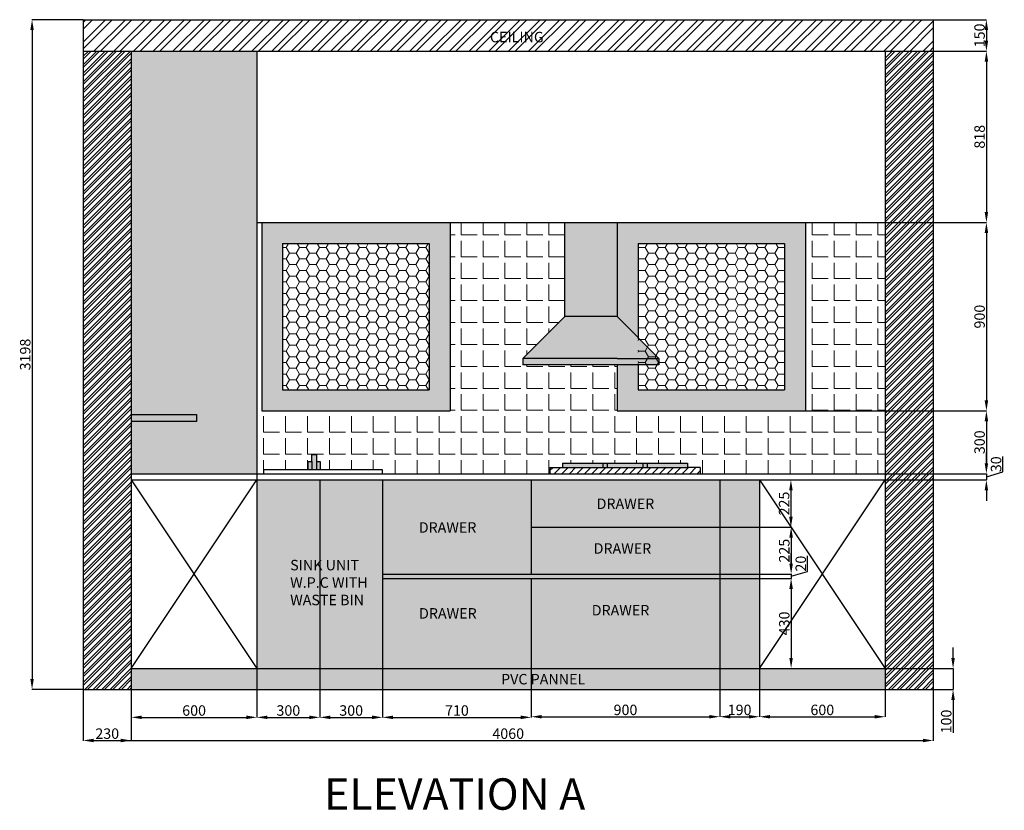
# Model space of a CAD drawing. Units: millimetres. Extents: x 4283 to 9420, y -2853 to 5191.
# Tile 1 of 2: x 4283 to 8985, y -2853 to 922. Entities that reach past the tile are written whole.
import ezdxf

# ---------------------------------------------------------------- set-up
doc = ezdxf.new("R2010")
doc.units = ezdxf.units.MM
for name, color, linetype, lineweight in [('A-ANNO-DIMS', 2, 'Continuous', 18), ('A-ANNO-TEXT', 7, 'Continuous', 18), ('A-ELEV', 7, 'Continuous', 25), ('A-ELEV-PATT', 252, 'Continuous', 13)]:
    doc.layers.add(name, color=color, linetype=linetype, lineweight=lineweight)
doc.styles.get("Standard").update_dxf_attribs({"font": 'arial.ttf'})
doc.dimstyles.new('ISO-25', dxfattribs={"dimtxt": 50, "dimasz": 50, "dimexe": 1.25, "dimexo": 0.625, "dimtad": 1, "dimdec": 0, "dimtxsty": 'Standard', "dimcen": 2.5, "dimclrd": 4, "dimclre": 4, "dimclrt": 4, "dimadec": 0, "dimazin": 0, "dimtfac": 1, "dimtdec": 0, "dimtmove": 0, "dimatfit": 3, "dimfxl": 1, "dimarcsym": 0})

# ---------------------------------------------------------------- blocks, each defined once
blk = doc.blocks.new('*D20')
at = {"layer": 'A-ANNO-DIMS', "color": 0, "lineweight": -2, "transparency": 16777216}
for p, q in [((8647.1, 922.3), (8901.2, 922.3)), ((8900, 872.3), (8900, 822.3)), ((8647.1, 772.3), (8901.2, 772.3))]:
    blk.add_line(p, q, dxfattribs=at)
at = {"layer": 'A-ANNO-DIMS', "color": 0, "transparency": 16777216}
for points in [[(8891.7, 872.3), (8908.3, 872.3), (8900, 922.3)], [(8891.7, 822.3), (8908.3, 822.3), (8900, 772.3)]]:
    blk.add_solid(points, dxfattribs=at)
at = {"layer": 'Defpoints', "color": 0, "transparency": 16777216}
for p in [(8646.4, 922.3), (8646.4, 772.3), (8900, 772.3)]:
    blk.add_point(p, dxfattribs=at)
at = {"layer": 'A-ANNO-DIMS', "color": 0, "transparency": 16777216, "insert": (8873.8, 847.3), "char_height": 50, "attachment_point": 5, "rotation": 90}
blk.add_mtext('150', dxfattribs=at)
blk = doc.blocks.new('*D21')
at = {"layer": 'A-ANNO-DIMS', "color": 0, "lineweight": -2, "transparency": 16777216}
for p, q in [((8647.1, 772.3), (8901.2, 772.3)), ((8900, 722.3), (8900, 4.3)), ((8417.1, -45.7), (8901.2, -45.7))]:
    blk.add_line(p, q, dxfattribs=at)
at = {"layer": 'A-ANNO-DIMS', "color": 0, "transparency": 16777216}
for points in [[(8891.7, 722.3), (8908.3, 722.3), (8900, 772.3)], [(8891.7, 4.3), (8908.3, 4.3), (8900, -45.7)]]:
    blk.add_solid(points, dxfattribs=at)
at = {"layer": 'Defpoints', "color": 0, "transparency": 16777216}
for p in [(8646.4, 772.3), (8416.4, -45.7), (8900, -45.7)]:
    blk.add_point(p, dxfattribs=at)
at = {"layer": 'A-ANNO-DIMS', "color": 0, "transparency": 16777216, "insert": (8873.8, 363.3), "char_height": 50, "attachment_point": 5, "rotation": 90}
blk.add_mtext('818', dxfattribs=at)
blk = doc.blocks.new('*D22')
at = {"layer": 'A-ANNO-DIMS', "color": 0, "lineweight": -2, "transparency": 16777216}
for p, q in [((8417.1, -45.7), (8901.2, -45.7)), ((8900, -95.7), (8900, -895.7)), ((8036.9, -945.7), (8901.2, -945.7))]:
    blk.add_line(p, q, dxfattribs=at)
at = {"layer": 'A-ANNO-DIMS', "color": 0, "transparency": 16777216}
for points in [[(8891.7, -95.7), (8908.3, -95.7), (8900, -45.7)], [(8891.7, -895.7), (8908.3, -895.7), (8900, -945.7)]]:
    blk.add_solid(points, dxfattribs=at)
at = {"layer": 'Defpoints', "color": 0, "transparency": 16777216}
for p in [(8416.4, -45.7), (8036.3, -945.7), (8900, -945.7)]:
    blk.add_point(p, dxfattribs=at)
at = {"layer": 'A-ANNO-DIMS', "color": 0, "transparency": 16777216, "insert": (8873.8, -495.7), "char_height": 50, "attachment_point": 5, "rotation": 90}
blk.add_mtext('900', dxfattribs=at)
blk = doc.blocks.new('*D23')
at = {"layer": 'A-ANNO-DIMS', "color": 0, "lineweight": -2, "transparency": 16777216}
for p, q in [((8036.9, -945.7), (8901.2, -945.7)), ((8900, -995.7), (8900, -1195.7)), ((8417.1, -1245.7), (8901.2, -1245.7))]:
    blk.add_line(p, q, dxfattribs=at)
at = {"layer": 'A-ANNO-DIMS', "color": 0, "transparency": 16777216}
for points in [[(8891.7, -995.7), (8908.3, -995.7), (8900, -945.7)], [(8891.7, -1195.7), (8908.3, -1195.7), (8900, -1245.7)]]:
    blk.add_solid(points, dxfattribs=at)
at = {"layer": 'Defpoints', "color": 0, "transparency": 16777216}
for p in [(8036.3, -945.7), (8416.4, -1245.7), (8900, -1245.7)]:
    blk.add_point(p, dxfattribs=at)
at = {"layer": 'A-ANNO-DIMS', "color": 0, "transparency": 16777216, "insert": (8873.8, -1095.7), "char_height": 50, "attachment_point": 5, "rotation": 90}
blk.add_mtext('300', dxfattribs=at)
blk = doc.blocks.new('*D24')
at = {"layer": 'A-ANNO-DIMS', "color": 0, "lineweight": -2, "transparency": 16777216}
for p, q in [((8900, -1195.7), (8900, -1145.7)), ((8978.8, -1237.1), (8978.8, -1164.4)), ((8417.1, -1245.7), (8901.2, -1245.7)), ((8900, -1260.7), (8978.8, -1237.1)), ((8900, -1245.7), (8900, -1275.7)), ((8900, -1245.7), (8900, -1275.7)), ((8417.1, -1275.7), (8901.2, -1275.7)), ((8900, -1325.7), (8900, -1375.7))]:
    blk.add_line(p, q, dxfattribs=at)
at = {"layer": 'A-ANNO-DIMS', "color": 0, "transparency": 16777216}
for points in [[(8891.7, -1195.7), (8908.3, -1195.7), (8900, -1245.7)], [(8891.7, -1325.7), (8908.3, -1325.7), (8900, -1275.7)]]:
    blk.add_solid(points, dxfattribs=at)
at = {"layer": 'Defpoints', "color": 0, "transparency": 16777216}
for p in [(8416.4, -1245.7), (8416.4, -1275.7), (8900, -1275.7)]:
    blk.add_point(p, dxfattribs=at)
at = {"layer": 'A-ANNO-DIMS', "color": 0, "transparency": 16777216, "insert": (8952.7, -1200.8), "char_height": 50, "attachment_point": 5, "rotation": 90}
blk.add_mtext('30', dxfattribs=at)
blk = doc.blocks.new('*D25')
at = {"layer": 'A-ANNO-DIMS', "color": 0, "lineweight": -2, "transparency": 16777216}
for p, q in [((8740.8, -2125.7), (8740.8, -2075.7)), ((8417.1, -2175.7), (8742, -2175.7)), ((8740.8, -2175.7), (8740.8, -2275.7)), ((8417.1, -2275.7), (8742, -2275.7)), ((8740.8, -2325.7), (8740.8, -2482.6))]:
    blk.add_line(p, q, dxfattribs=at)
at = {"layer": 'A-ANNO-DIMS', "color": 0, "transparency": 16777216}
for points in [[(8732.5, -2125.7), (8749.1, -2125.7), (8740.8, -2175.7)], [(8732.5, -2325.7), (8749.1, -2325.7), (8740.8, -2275.7)]]:
    blk.add_solid(points, dxfattribs=at)
at = {"layer": 'Defpoints', "color": 0, "transparency": 16777216}
for p in [(8416.4, -2175.7), (8416.4, -2275.7), (8740.8, -2275.7)]:
    blk.add_point(p, dxfattribs=at)
at = {"layer": 'A-ANNO-DIMS', "color": 0, "transparency": 16777216, "insert": (8714.6, -2429.2), "char_height": 50, "attachment_point": 5, "rotation": 90}
blk.add_mtext('100', dxfattribs=at)
blk = doc.blocks.new('*D26')
at = {"layer": 'A-ANNO-DIMS', "color": 0, "lineweight": -2, "transparency": 16777216}
for p, q in [((4816.4, -2176.4), (4816.4, -2410.5)), ((5416.4, -2176.4), (5416.4, -2410.5)), ((4866.4, -2409.3), (5366.4, -2409.3))]:
    blk.add_line(p, q, dxfattribs=at)
at = {"layer": 'A-ANNO-DIMS', "color": 0, "transparency": 16777216}
for points in [[(4866.4, -2400.9), (4866.4, -2417.6), (4816.4, -2409.3)], [(5366.4, -2400.9), (5366.4, -2417.6), (5416.4, -2409.3)]]:
    blk.add_solid(points, dxfattribs=at)
at = {"layer": 'Defpoints', "color": 0, "transparency": 16777216}
for p in [(4816.4, -2175.7), (5416.4, -2175.7), (5416.4, -2409.3)]:
    blk.add_point(p, dxfattribs=at)
at = {"layer": 'A-ANNO-DIMS', "color": 0, "transparency": 16777216, "insert": (5116.4, -2383.1), "char_height": 50, "attachment_point": 5}
blk.add_mtext('600', dxfattribs=at)
blk = doc.blocks.new('*D27')
at = {"layer": 'A-ANNO-DIMS', "color": 0, "lineweight": -2, "transparency": 16777216}
for p, q in [((5416.4, -2176.4), (5416.4, -2410.5)), ((5716.4, -2176.4), (5716.4, -2410.5)), ((5466.4, -2409.3), (5666.4, -2409.3))]:
    blk.add_line(p, q, dxfattribs=at)
at = {"layer": 'A-ANNO-DIMS', "color": 0, "transparency": 16777216}
for points in [[(5466.4, -2400.9), (5466.4, -2417.6), (5416.4, -2409.3)], [(5666.4, -2400.9), (5666.4, -2417.6), (5716.4, -2409.3)]]:
    blk.add_solid(points, dxfattribs=at)
at = {"layer": 'Defpoints', "color": 0, "transparency": 16777216}
for p in [(5416.4, -2175.7), (5716.4, -2175.7), (5716.4, -2409.3)]:
    blk.add_point(p, dxfattribs=at)
at = {"layer": 'A-ANNO-DIMS', "color": 0, "transparency": 16777216, "insert": (5566.4, -2383.1), "char_height": 50, "attachment_point": 5}
blk.add_mtext('300', dxfattribs=at)
blk = doc.blocks.new('*D28')
at = {"layer": 'A-ANNO-DIMS', "color": 0, "lineweight": -2, "transparency": 16777216}
for p, q in [((5716.4, -2176.4), (5716.4, -2410.5)), ((6016.4, -2176.4), (6016.4, -2410.5)), ((5766.4, -2409.3), (5966.4, -2409.3))]:
    blk.add_line(p, q, dxfattribs=at)
at = {"layer": 'A-ANNO-DIMS', "color": 0, "transparency": 16777216}
for points in [[(5766.4, -2400.9), (5766.4, -2417.6), (5716.4, -2409.3)], [(5966.4, -2400.9), (5966.4, -2417.6), (6016.4, -2409.3)]]:
    blk.add_solid(points, dxfattribs=at)
at = {"layer": 'Defpoints', "color": 0, "transparency": 16777216}
for p in [(5716.4, -2175.7), (6016.4, -2175.7), (6016.4, -2409.3)]:
    blk.add_point(p, dxfattribs=at)
at = {"layer": 'A-ANNO-DIMS', "color": 0, "transparency": 16777216, "insert": (5866.4, -2383.1), "char_height": 50, "attachment_point": 5}
blk.add_mtext('300', dxfattribs=at)
blk = doc.blocks.new('*D29')
at = {"layer": 'A-ANNO-DIMS', "color": 0, "lineweight": -2, "transparency": 16777216}
for p, q in [((6016.4, -2176.4), (6016.4, -2410.5)), ((6726.4, -2176.4), (6726.4, -2410.5)), ((6066.4, -2409.3), (6676.4, -2409.3))]:
    blk.add_line(p, q, dxfattribs=at)
at = {"layer": 'A-ANNO-DIMS', "color": 0, "transparency": 16777216}
for points in [[(6066.4, -2400.9), (6066.4, -2417.6), (6016.4, -2409.3)], [(6676.4, -2400.9), (6676.4, -2417.6), (6726.4, -2409.3)]]:
    blk.add_solid(points, dxfattribs=at)
at = {"layer": 'Defpoints', "color": 0, "transparency": 16777216}
for p in [(6016.4, -2175.7), (6726.4, -2175.7), (6726.4, -2409.3)]:
    blk.add_point(p, dxfattribs=at)
at = {"layer": 'A-ANNO-DIMS', "color": 0, "transparency": 16777216, "insert": (6371.4, -2383.1), "char_height": 50, "attachment_point": 5}
blk.add_mtext('710', dxfattribs=at)
blk = doc.blocks.new('*D30')
at = {"layer": 'A-ANNO-DIMS', "color": 0, "lineweight": -2, "transparency": 16777216}
for p, q in [((6726.4, -2176.4), (6726.4, -2407.6)), ((7626.4, -2176.4), (7626.4, -2407.6)), ((6776.4, -2406.3), (7576.4, -2406.3))]:
    blk.add_line(p, q, dxfattribs=at)
at = {"layer": 'A-ANNO-DIMS', "color": 0, "transparency": 16777216}
for points in [[(6776.4, -2398), (6776.4, -2414.7), (6726.4, -2406.3)], [(7576.4, -2398), (7576.4, -2414.7), (7626.4, -2406.3)]]:
    blk.add_solid(points, dxfattribs=at)
at = {"layer": 'Defpoints', "color": 0, "transparency": 16777216}
for p in [(6726.4, -2175.7), (7626.4, -2175.7), (7626.4, -2406.3)]:
    blk.add_point(p, dxfattribs=at)
at = {"layer": 'A-ANNO-DIMS', "color": 0, "transparency": 16777216, "insert": (7176.4, -2380.2), "char_height": 50, "attachment_point": 5}
blk.add_mtext('900', dxfattribs=at)
blk = doc.blocks.new('*D31')
at = {"layer": 'A-ANNO-DIMS', "color": 0, "lineweight": -2, "transparency": 16777216}
for p, q in [((7626.4, -2176.4), (7626.4, -2407.6)), ((7816.4, -2176.4), (7816.4, -2407.6)), ((7676.4, -2406.3), (7766.4, -2406.3))]:
    blk.add_line(p, q, dxfattribs=at)
at = {"layer": 'A-ANNO-DIMS', "color": 0, "transparency": 16777216}
for points in [[(7676.4, -2398), (7676.4, -2414.7), (7626.4, -2406.3)], [(7766.4, -2398), (7766.4, -2414.7), (7816.4, -2406.3)]]:
    blk.add_solid(points, dxfattribs=at)
at = {"layer": 'Defpoints', "color": 0, "transparency": 16777216}
for p in [(7626.4, -2175.7), (7816.4, -2175.7), (7816.4, -2406.3)]:
    blk.add_point(p, dxfattribs=at)
at = {"layer": 'A-ANNO-DIMS', "color": 0, "transparency": 16777216, "insert": (7721.4, -2380.2), "char_height": 50, "attachment_point": 5}
blk.add_mtext('190', dxfattribs=at)
blk = doc.blocks.new('*D32')
at = {"layer": 'A-ANNO-DIMS', "color": 0, "lineweight": -2, "transparency": 16777216}
for p, q in [((7816.4, -2176.4), (7816.4, -2407.6)), ((8416.4, -2176.4), (8416.4, -2407.6)), ((7866.4, -2406.3), (8366.4, -2406.3))]:
    blk.add_line(p, q, dxfattribs=at)
at = {"layer": 'A-ANNO-DIMS', "color": 0, "transparency": 16777216}
for points in [[(7866.4, -2398), (7866.4, -2414.7), (7816.4, -2406.3)], [(8366.4, -2398), (8366.4, -2414.7), (8416.4, -2406.3)]]:
    blk.add_solid(points, dxfattribs=at)
at = {"layer": 'Defpoints', "color": 0, "transparency": 16777216}
for p in [(7816.4, -2175.7), (8416.4, -2175.7), (8416.4, -2406.3)]:
    blk.add_point(p, dxfattribs=at)
at = {"layer": 'A-ANNO-DIMS', "color": 0, "transparency": 16777216, "insert": (8116.4, -2380.2), "char_height": 50, "attachment_point": 5}
blk.add_mtext('600', dxfattribs=at)
blk = doc.blocks.new('*D33')
at = {"layer": 'A-ANNO-DIMS', "color": 0, "lineweight": -2, "transparency": 16777216}
for p, q in [((7627.1, -1275.7), (7967.7, -1275.7)), ((7966.4, -1325.7), (7966.4, -1450.7)), ((7627.1, -1500.7), (7967.7, -1500.7))]:
    blk.add_line(p, q, dxfattribs=at)
at = {"layer": 'A-ANNO-DIMS', "color": 0, "transparency": 16777216}
for points in [[(7958.1, -1325.7), (7974.8, -1325.7), (7966.4, -1275.7)], [(7958.1, -1450.7), (7974.8, -1450.7), (7966.4, -1500.7)]]:
    blk.add_solid(points, dxfattribs=at)
at = {"layer": 'Defpoints', "color": 0, "transparency": 16777216}
for p in [(7626.4, -1275.7), (7626.4, -1500.7), (7966.4, -1500.7)]:
    blk.add_point(p, dxfattribs=at)
at = {"layer": 'A-ANNO-DIMS', "color": 0, "transparency": 16777216, "insert": (7940.3, -1388.2), "char_height": 50, "attachment_point": 5, "rotation": 90}
blk.add_mtext('225', dxfattribs=at)
blk = doc.blocks.new('*D34')
at = {"layer": 'A-ANNO-DIMS', "color": 0, "lineweight": -2, "transparency": 16777216}
for p, q in [((7627.1, -1500.7), (7968.6, -1500.7)), ((7967.4, -1550.7), (7967.4, -1675.7)), ((7627.1, -1725.7), (7968.6, -1725.7))]:
    blk.add_line(p, q, dxfattribs=at)
at = {"layer": 'A-ANNO-DIMS', "color": 0, "transparency": 16777216}
for points in [[(7959, -1550.7), (7975.7, -1550.7), (7967.4, -1500.7)], [(7959, -1675.7), (7975.7, -1675.7), (7967.4, -1725.7)]]:
    blk.add_solid(points, dxfattribs=at)
at = {"layer": 'Defpoints', "color": 0, "transparency": 16777216}
for p in [(7626.4, -1500.7), (7626.4, -1725.7), (7967.4, -1725.7)]:
    blk.add_point(p, dxfattribs=at)
at = {"layer": 'A-ANNO-DIMS', "color": 0, "transparency": 16777216, "insert": (7941.2, -1613.2), "char_height": 50, "attachment_point": 5, "rotation": 90}
blk.add_mtext('225', dxfattribs=at)
blk = doc.blocks.new('*D35')
at = {"layer": 'A-ANNO-DIMS', "color": 0, "lineweight": -2, "transparency": 16777216}
for p, q in [((7967.4, -1675.7), (7967.4, -1625.7)), ((8046.2, -1712.1), (8046.2, -1638.6)), ((7627.1, -1725.7), (7968.6, -1725.7)), ((7967.4, -1735.7), (8046.2, -1712.1)), ((7967.4, -1725.7), (7967.4, -1745.7)), ((7967.4, -1725.7), (7967.4, -1745.7)), ((7627.1, -1745.7), (7968.6, -1745.7)), ((7967.4, -1795.7), (7967.4, -1845.7))]:
    blk.add_line(p, q, dxfattribs=at)
at = {"layer": 'A-ANNO-DIMS', "color": 0, "transparency": 16777216}
for points in [[(7959, -1675.7), (7975.7, -1675.7), (7967.4, -1725.7)], [(7959, -1795.7), (7975.7, -1795.7), (7967.4, -1745.7)]]:
    blk.add_solid(points, dxfattribs=at)
at = {"layer": 'Defpoints', "color": 0, "transparency": 16777216}
for p in [(7626.4, -1725.7), (7626.4, -1745.7), (7967.4, -1745.7)]:
    blk.add_point(p, dxfattribs=at)
at = {"layer": 'A-ANNO-DIMS', "color": 0, "transparency": 16777216, "insert": (8020, -1675.3), "char_height": 50, "attachment_point": 5, "rotation": 90}
blk.add_mtext('20', dxfattribs=at)
blk = doc.blocks.new('*D36')
at = {"layer": 'A-ANNO-DIMS', "color": 0, "lineweight": -2, "transparency": 16777216}
for p, q in [((7627.1, -1745.7), (7968.6, -1745.7)), ((7967.4, -1795.7), (7967.4, -2125.7)), ((7627.1, -2175.7), (7968.6, -2175.7))]:
    blk.add_line(p, q, dxfattribs=at)
at = {"layer": 'A-ANNO-DIMS', "color": 0, "transparency": 16777216}
for points in [[(7959, -1795.7), (7975.7, -1795.7), (7967.4, -1745.7)], [(7959, -2125.7), (7975.7, -2125.7), (7967.4, -2175.7)]]:
    blk.add_solid(points, dxfattribs=at)
at = {"layer": 'Defpoints', "color": 0, "transparency": 16777216}
for p in [(7626.4, -1745.7), (7626.4, -2175.7), (7967.4, -2175.7)]:
    blk.add_point(p, dxfattribs=at)
at = {"layer": 'A-ANNO-DIMS', "color": 0, "transparency": 16777216, "insert": (7941.2, -1960.7), "char_height": 50, "attachment_point": 5, "rotation": 90}
blk.add_mtext('430', dxfattribs=at)
blk = doc.blocks.new('*D50')
at = {"layer": 'A-ANNO-DIMS', "color": 4, "lineweight": -2, "transparency": 16777216}
for p, q in [((4586.4, -2276.4), (4586.4, -2521)), ((4816.4, -2276.4), (4816.4, -2521)), ((4636.4, -2519.7), (4766.4, -2519.7))]:
    blk.add_line(p, q, dxfattribs=at)
at = {"layer": 'A-ANNO-DIMS', "color": 4, "transparency": 16777216}
for points in [[(4636.4, -2511.4), (4636.4, -2528.1), (4586.4, -2519.7)], [(4766.4, -2511.4), (4766.4, -2528.1), (4816.4, -2519.7)]]:
    blk.add_solid(points, dxfattribs=at)
at = {"layer": 'Defpoints', "color": 0, "transparency": 16777216}
for p in [(4586.4, -2275.7), (4816.4, -2275.7), (4816.4, -2519.7)]:
    blk.add_point(p, dxfattribs=at)
at = {"layer": 'A-ANNO-DIMS', "color": 4, "transparency": 16777216, "insert": (4701.4, -2493.6), "char_height": 50, "attachment_point": 5}
blk.add_mtext('230', dxfattribs=at)
blk = doc.blocks.new('*D51')
at = {"layer": 'A-ANNO-DIMS', "color": 4, "lineweight": -2, "transparency": 16777216}
for p, q in [((4586.4, -2276.4), (4586.4, -2521)), ((8646.4, -2276.4), (8646.4, -2521)), ((4636.4, -2519.7), (8596.4, -2519.7))]:
    blk.add_line(p, q, dxfattribs=at)
at = {"layer": 'A-ANNO-DIMS', "color": 4, "transparency": 16777216}
for points in [[(4636.4, -2511.4), (4636.4, -2528.1), (4586.4, -2519.7)], [(8596.4, -2511.4), (8596.4, -2528.1), (8646.4, -2519.7)]]:
    blk.add_solid(points, dxfattribs=at)
at = {"layer": 'Defpoints', "color": 0, "transparency": 16777216}
for p in [(4586.4, -2275.7), (8646.4, -2275.7), (8646.4, -2519.7)]:
    blk.add_point(p, dxfattribs=at)
at = {"layer": 'A-ANNO-DIMS', "color": 4, "transparency": 16777216, "insert": (6616.4, -2493.6), "char_height": 50, "attachment_point": 5}
blk.add_mtext('4060', dxfattribs=at)
blk = doc.blocks.new('*D52')
at = {"layer": 'A-ANNO-DIMS', "color": 4, "lineweight": -2, "transparency": 16777216}
for p, q in [((4585.8, 922.3), (4341.2, 922.3)), ((4342.4, 872.3), (4342.4, -2225.7)), ((4585.8, -2275.7), (4341.2, -2275.7))]:
    blk.add_line(p, q, dxfattribs=at)
at = {"layer": 'A-ANNO-DIMS', "color": 4, "transparency": 16777216}
for points in [[(4334.1, 872.3), (4350.8, 872.3), (4342.4, 922.3)], [(4334.1, -2225.7), (4350.8, -2225.7), (4342.4, -2275.7)]]:
    blk.add_solid(points, dxfattribs=at)
at = {"layer": 'Defpoints', "color": 0, "transparency": 16777216}
for p in [(4586.4, 922.3), (4342.4, -2275.7), (4586.4, -2275.7)]:
    blk.add_point(p, dxfattribs=at)
at = {"layer": 'A-ANNO-DIMS', "color": 4, "transparency": 16777216, "insert": (4316.3, -676.7), "char_height": 50, "attachment_point": 5, "rotation": 90}
blk.add_mtext('3198', dxfattribs=at)

msp = doc.modelspace()

# ---------------------------------------------------------------- hatches: boundary and pattern name
at = {"layer": 'A-ELEV-PATT'}
h = msp.add_hatch(dxfattribs=at)
h.set_pattern_fill('ANSI32', color=256, scale=7)
h.paths.add_polyline_path([(8646.43, 922.26), (4586.43, 922.26), (4586.43, 772.26), (8646.43, 772.26)])
h = msp.add_hatch(dxfattribs=at)
h.set_pattern_fill('ANSI32', color=256, scale=3)
h.paths.add_polyline_path([(4816.43, 772.26), (4586.43, 772.26), (4586.43, -2275.74), (4816.43, -2275.74)])
h.paths.add_polyline_path([(8646.43, 772.26), (8416.43, 772.26), (8416.43, -2275.74), (8646.43, -2275.74)])
h = msp.add_hatch(color=256, dxfattribs=at)
h.dxf.hatch_style = 1
h.paths.add_polyline_path([(5416.43, 772.26), (4816.43, 772.26), (4816.43, -962.54), (5128.05, -962.54), (5128.05, -997.25), (4816.43, -997.25), (4816.43, -1245.74), (5416.43, -1245.74)])
h = msp.add_hatch(dxfattribs=at)
h.set_pattern_fill('ANGLE', color=256, scale=15)
h.set_pattern_definition([(0, (0, 0), (0, 104.775), [76.2, -28.575]), (90, (0, 0), (-104.775, 6e-15), [76.2, -28.575])])
h.paths.add_polyline_path([(6886.26, -45.74), (6339.12, -45.74), (6339.12, -945.74), (5439.12, -945.74), (5439.12, -45.74), (5416.43, -45.74), (5416.43, -1245.74), (5447.13, -1245.74), (5447.13, -1225.74), (5660.96, -1225.74), (5660.96, -1187.34), (5678.56, -1187.34), (5678.56, -1153.92), (5701.44, -1153.92), (5701.44, -1187.34), (5719.04, -1187.34), (5719.04, -1225.74), (6014.01, -1225.74), (6014.01, -1245.74), (6815.51, -1245.74), (6815.51, -1215.74), (6875.56, -1215.74), (6875.56, -1195.74), (7472.53, -1195.74), (7472.53, -1215.74), (7532.58, -1215.74), (7532.58, -1245.74), (8416.43, -1245.74), (8416.43, -45.74), (8036.26, -45.74), (8036.26, -945.74), (7136.26, -945.74), (7136.26, -725.74), (6686.26, -725.74), (6686.26, -695.74), (6886.26, -495.74)])
h = msp.add_hatch(color=256, dxfattribs=at)
h.dxf.hatch_style = 1
h.paths.add_polyline_path([(6339.12, -45.74), (5439.12, -45.74), (5439.12, -945.74), (6339.12, -945.74)])
h.paths.add_polyline_path([(5539.12, -845.74), (5539.12, -145.74), (6239.12, -145.74), (6239.12, -845.74)], flags=16)
h.paths.add_polyline_path([(8036.26, -45.74), (7136.26, -45.74), (7136.26, -945.74), (8036.26, -945.74)])
h.paths.add_polyline_path([(7236.26, -845.74), (7236.26, -145.74), (7936.26, -145.74), (7936.26, -845.74)], flags=16)
h = msp.add_hatch(color=256, dxfattribs=at)
h.dxf.hatch_style = 1
h.paths.add_polyline_path([(7136.26, -45.74), (6886.26, -45.74), (6886.26, -495.74), (7136.26, -495.74)])
h.paths.add_polyline_path([(7136.26, -495.74), (6886.26, -495.74), (6686.26, -695.74), (6886.26, -695.74), (7136.26, -695.74)])
h.paths.add_polyline_path([(7136.26, -695.74), (6886.26, -695.74), (6686.26, -695.74), (6686.26, -725.74), (7136.26, -725.74)])
h.paths.add_polyline_path([(7336.26, -695.74), (7236.26, -695.74), (7236.26, -725.74), (7336.26, -725.74)])
h.paths.add_polyline_path([(7236.26, -595.74), (7136.26, -495.74), (7136.26, -695.74), (7236.26, -695.74)])
h.paths.add_polyline_path([(7236.26, -695.74), (7136.26, -695.74), (7136.26, -725.74), (7236.26, -725.74)])
h.paths.add_polyline_path([(7236.26, -595.74), (7236.26, -695.74), (7336.26, -695.74)])
h = msp.add_hatch(dxfattribs=at)
h.set_pattern_fill('HONEY', color=256, scale=10)
h.paths.add_polyline_path([(6239.12, -145.74), (5539.12, -145.74), (5539.12, -845.74), (6239.12, -845.74)])
h.paths.add_polyline_path([(7936.26, -145.74), (7236.26, -145.74), (7236.26, -845.74), (7936.26, -845.74)])
h = msp.add_hatch(color=256, dxfattribs=at)
h.dxf.hatch_style = 1
h.paths.add_polyline_path([(5128.05, -962.54), (4816.43, -962.54), (4816.43, -997.25), (5128.05, -997.25)])
h = msp.add_hatch(color=256, dxfattribs=at)
h.dxf.hatch_style = 1
h.paths.add_polyline_path([(7088.5, -1195.74), (7068.08, -1195.74), (7068.08, -1215.74), (7088.5, -1215.74)])
h.paths.add_polyline_path([(7280.02, -1195.74), (7259.59, -1195.74), (7259.59, -1215.74), (7280.02, -1215.74)])
h.paths.add_polyline_path([(5701.44, -1153.92), (5678.56, -1153.92), (5678.56, -1187.34), (5678.56, -1225.74), (5701.44, -1225.74)])
h.paths.add_polyline_path([(5719.04, -1187.34), (5701.44, -1187.34), (5701.44, -1225.74), (5719.04, -1225.74)])
h.paths.add_polyline_path([(5678.56, -1187.34), (5660.96, -1187.34), (5660.96, -1225.74), (5678.56, -1225.74)])
h = msp.add_hatch(dxfattribs=at)
h.set_pattern_fill('ANSI31', color=256, scale=8)
h.paths.add_polyline_path([(7532.58, -1215.74), (7472.53, -1215.74), (6875.56, -1215.74), (6815.51, -1215.74), (6815.51, -1245.74), (7532.58, -1245.74)])
h = msp.add_hatch(color=256, dxfattribs=at)
h.dxf.hatch_style = 1
h.paths.add_polyline_path([(7472.53, -1195.74), (7280.02, -1195.74), (7280.02, -1215.74), (7472.53, -1215.74)])
h.paths.add_polyline_path([(7259.59, -1195.74), (7088.5, -1195.74), (7088.5, -1215.74), (7259.59, -1215.74)])
h.paths.add_polyline_path([(7068.08, -1195.74), (6875.56, -1195.74), (6875.56, -1215.74), (7068.08, -1215.74)])
h = msp.add_hatch(color=256, dxfattribs=at)
h.dxf.hatch_style = 1
h.paths.add_polyline_path([(5716.43, -1275.74), (5416.43, -1275.74), (5416.43, -2175.74), (5716.43, -2175.74)])
h.paths.add_polyline_path([(6016.43, -1275.74), (5716.43, -1275.74), (5716.43, -2175.74), (6016.43, -2175.74)])
h.paths.add_polyline_path([(6726.43, -1275.74), (6016.43, -1275.74), (6016.43, -1725.74), (6726.43, -1725.74)])
h.paths.add_polyline_path([(6726.43, -1745.74), (6016.43, -1745.74), (6016.43, -2175.74), (6726.43, -2175.74)])
h.paths.add_polyline_path([(7626.43, -1275.74), (6726.43, -1275.74), (6726.43, -1500.74), (7626.43, -1500.74)])
h.paths.add_polyline_path([(7626.43, -1500.74), (6726.43, -1500.74), (6726.43, -1725.74), (7626.43, -1725.74)])
h.paths.add_polyline_path([(7626.43, -1745.74), (6726.43, -1745.74), (6726.43, -2175.74), (7626.43, -2175.74)])
h.paths.add_polyline_path([(7816.43, -1275.74), (7626.43, -1275.74), (7626.43, -2175.74), (7816.43, -2175.74)])
h = msp.add_hatch(color=256, dxfattribs=at)
h.dxf.hatch_style = 1
h.paths.add_polyline_path([(6726.43, -1725.74), (6016.43, -1725.74), (6016.43, -1745.74), (6726.43, -1745.74)])
h.paths.add_polyline_path([(7626.43, -1725.74), (6726.43, -1725.74), (6726.43, -1745.74), (7626.43, -1745.74)])
h = msp.add_hatch(color=256, dxfattribs=at)
h.dxf.hatch_style = 1
h.paths.add_polyline_path([(8416.43, -2175.74), (4816.43, -2175.74), (4816.43, -2275.74), (8416.43, -2275.74)])

# ---------------------------------------------------------------- linework, layer by layer
at = {"layer": 'A-ELEV'}
for p, q in [((4586.43, 922.26), (8646.43, 922.26)), ((4586.43, 922.26), (4586.43, -2275.74)), ((8646.43, 922.26), (8646.43, -2275.74)), ((4586.43, 772.26), (8646.43, 772.26)), ((4816.43, 772.26), (4816.43, -2275.74)), ((5416.43, 772.26), (5416.43, -2175.74)), ((8416.43, 772.26), (8416.43, -2275.74)), ((5416.43, -45.74), (8416.43, -45.74)), ((5439.12, -45.74), (5439.12, -945.74)), ((6339.12, -45.74), (6339.12, -945.74)), ((6886.26, -495.74), (6886.26, -45.74)), ((7136.26, -45.74), (7136.26, -495.74)), ((7136.26, -45.74), (7136.26, -495.74)), ((8036.26, -45.74), (8036.26, -945.74)), ((5539.12, -145.74), (6239.12, -145.74)), ((5539.12, -145.74), (5539.12, -845.74)), ((6239.12, -145.74), (6239.12, -845.74)), ((7236.26, -145.74), (7236.26, -595.74)), ((7236.26, -145.74), (7936.26, -145.74)), ((7936.26, -145.74), (7936.26, -845.74)), ((6886.26, -495.74), (6686.26, -695.74)), ((7136.26, -495.74), (6886.26, -495.74)), ((7136.26, -495.74), (7336.26, -695.74)), ((6886.26, -695.74), (6686.26, -695.74)), ((6686.26, -695.74), (6686.26, -725.74)), ((7136.26, -695.74), (6886.26, -695.74)), ((7136.26, -695.74), (7336.26, -695.74)), ((7336.26, -695.74), (7336.26, -725.74)), ((7336.26, -725.74), (6686.26, -725.74)), ((7136.26, -725.74), (7136.26, -945.74)), ((7236.26, -725.74), (7236.26, -845.74)), ((5539.12, -845.74), (6239.12, -845.74)), ((7236.26, -845.74), (7936.26, -845.74)), ((4816.43, -962.54), (4816.43, -962.54)), ((4816.43, -962.54), (5128.05, -962.54)), ((5128.05, -962.54), (5128.05, -997.25)), ((5439.12, -945.74), (6339.12, -945.74)), ((7136.26, -945.74), (8036.26, -945.74)), ((5128.05, -997.25), (4816.43, -997.25)), ((5678.56, -1187.34), (5678.56, -1153.92)), ((5678.56, -1153.92), (5701.44, -1153.92)), ((5701.44, -1153.92), (5701.44, -1225.74)), ((5660.96, -1225.74), (5660.96, -1187.34)), ((5660.96, -1187.34), (5678.56, -1187.34)), ((5678.56, -1187.34), (5678.56, -1225.74)), ((5701.44, -1187.34), (5719.04, -1187.34)), ((5719.04, -1187.34), (5719.04, -1225.74)), ((6815.51, -1215.74), (6815.51, -1245.74)), ((6815.51, -1215.74), (6875.56, -1215.74)), ((6875.56, -1195.74), (7472.53, -1195.74)), ((6875.56, -1195.74), (6875.56, -1215.74)), ((6875.56, -1215.74), (7472.53, -1215.74)), ((7068.08, -1195.74), (7068.08, -1215.74)), ((7088.5, -1195.74), (7088.5, -1215.74)), ((7259.59, -1195.74), (7259.59, -1215.74)), ((7280.02, -1195.74), (7280.02, -1215.74)), ((7472.53, -1195.74), (7472.53, -1215.74)), ((7532.58, -1215.74), (7472.53, -1215.74)), ((7532.58, -1215.74), (7532.58, -1245.74)), ((4816.43, -1245.74), (8416.43, -1245.74)), ((5447.13, -1225.74), (5447.13, -1245.74)), ((5447.13, -1225.74), (6014.01, -1225.74)), ((6014.01, -1225.74), (6014.01, -1245.74)), ((4816.43, -1275.74), (8416.43, -1275.74)), ((4816.43, -2175.74), (5416.43, -1275.74)), ((4816.43, -1275.74), (5416.43, -2175.74)), ((5716.43, -1275.74), (5716.43, -2175.74)), ((6016.43, -1275.74), (6016.43, -2175.74)), ((6726.43, -1275.74), (6726.43, -1725.74)), ((7626.43, -1275.74), (7626.43, -2175.74)), ((7816.43, -1275.74), (7816.43, -2175.74)), ((7816.43, -2175.74), (8416.43, -1275.74)), ((7816.43, -1275.74), (8416.43, -2175.74)), ((6726.43, -1500.74), (7626.43, -1500.74)), ((6016.43, -1725.74), (7626.43, -1725.74)), ((6016.43, -1745.74), (7626.43, -1745.74)), ((6726.43, -1745.74), (6726.43, -2175.74)), ((4816.43, -2175.74), (8416.43, -2175.74)), ((4586.43, -2275.74), (8646.43, -2275.74))]:
    msp.add_line(p, q, dxfattribs=at)

# ---------------------------------------------------------------- texts
at = {"layer": 'A-ANNO-TEXT', "attachment_point": 1}
for s, width, insert, char_height in [('CEILING', 682.8521, (6529.09, 864.33), 50), ('DRAWER', 682.8521, (7038.56, -1364.31), 50), ('DRAWER', 682.8521, (6189.21, -1477.52), 50), ('DRAWER', 682.8521, (7024.24, -1577.92), 50), ('SINK UNIT\\PW.P.C WITH WASTE BIN', 563.2326, (5575.23, -1657.18), 50), ('DRAWER', 682.8521, (7015.19, -1872.85), 50), ('DRAWER', 682.8521, (6190.55, -1887.77), 50), ('PVC PANNEL', 682.8521, (6582.46, -2202.06), 50), ('{\\fArial|b1|i0|c0|p34;ELEVATION A}', 1908.7899, (5737.42, -2700.52), 150)]:
    msp.add_mtext_dynamic_manual_height_columns(s, width=width, gutter_width=12.5, heights=[0], dxfattribs=dict(at, insert=insert, char_height=char_height))

# ---------------------------------------------------------------- dimensions: what is measured, and where the dimension line sits
at = {"layer": 'A-ANNO-DIMS'}
for base, p1, p2, override, picture, middle in [((4342.43, -2275.74), (4586.43, 922.26), (4586.43, -2275.74), {"dimdec": 0, "dimlfac": 1, "dimrnd": 0, "dimzin": 0, "dimdsep": 46, "dimlunit": 2}, '*D52', (4316.26, -676.74)), ((8900, 772.26), (8646.43, 922.26), (8646.43, 772.26), {"dimclrd": 0, "dimclre": 0, "dimclrt": 0}, '*D20', (8873.85, 847.26)), ((8900, -45.74), (8646.43, 772.26), (8416.43, -45.74), {"dimclrd": 0, "dimclre": 0, "dimclrt": 0, "dimtmove": 1}, '*D21', (8873.85, 363.26)), ((8900, -945.74), (8416.43, -45.74), (8036.26, -945.74), {"dimclrd": 0, "dimclre": 0, "dimclrt": 0, "dimtmove": 1}, '*D22', (8873.85, -495.74)), ((8900, -1245.74), (8036.26, -945.74), (8416.43, -1245.74), {"dimclrd": 0, "dimclre": 0, "dimclrt": 0, "dimtmove": 1}, '*D23', (8873.83, -1095.74)), ((8900, -1275.74), (8416.43, -1245.74), (8416.43, -1275.74), {"dimclrd": 0, "dimclre": 0, "dimclrt": 0, "dimtmove": 1}, '*D24', (8952.65, -1236.47)), ((7966.43, -1500.74), (7626.43, -1275.74), (7626.43, -1500.74), {"dimclrd": 0, "dimclre": 0, "dimclrt": 0}, '*D33', (7940.28, -1388.24)), ((7967.38, -1725.74), (7626.43, -1500.74), (7626.43, -1725.74), {"dimclrd": 0, "dimclre": 0, "dimclrt": 0}, '*D34', (7941.23, -1613.24)), ((7967.38, -1745.74), (7626.43, -1725.74), (7626.43, -1745.74), {"dimclrd": 0, "dimclre": 0, "dimclrt": 0, "dimtmove": 1}, '*D35', (8020, -1711.49)), ((7967.38, -2175.74), (7626.43, -1745.74), (7626.43, -2175.74), {"dimclrd": 0, "dimclre": 0, "dimclrt": 0, "dimtmove": 1}, '*D36', (7941.21, -1960.74)), ((8740.8, -2275.74), (8416.43, -2175.74), (8416.43, -2275.74), {"dimclrd": 0, "dimclre": 0, "dimclrt": 0}, '*D25', (8714.64, -2429.17))]:
    dim = msp.add_linear_dim(base=base, p1=p1, p2=p2, angle=90, dimstyle='ISO-25', override=override, dxfattribs=at)
    dim.commit()
    dim.dimension.update_dxf_attribs({"geometry": picture, "text_midpoint": middle})
for base, p1, p2, override, picture, middle in [((5416.43, -2409.25), (4816.43, -2175.74), (5416.43, -2175.74), {"dimclrd": 0, "dimclre": 0, "dimclrt": 0}, '*D26', (5116.43, -2383.1)), ((5716.43, -2409.25), (5416.43, -2175.74), (5716.43, -2175.74), {"dimclrd": 0, "dimclre": 0, "dimclrt": 0, "dimtmove": 1}, '*D27', (5566.43, -2383.08)), ((6016.43, -2409.25), (5716.43, -2175.74), (6016.43, -2175.74), {"dimclrd": 0, "dimclre": 0, "dimclrt": 0, "dimtmove": 1}, '*D28', (5866.43, -2383.08)), ((6726.43, -2409.25), (6016.43, -2175.74), (6726.43, -2175.74), {"dimclrd": 0, "dimclre": 0, "dimclrt": 0, "dimtmove": 1}, '*D29', (6371.43, -2383.1)), ((7626.43, -2406.32), (6726.43, -2175.74), (7626.43, -2175.74), {"dimclrd": 0, "dimclre": 0, "dimclrt": 0}, '*D30', (7176.43, -2380.17)), ((7816.43, -2406.32), (7626.43, -2175.74), (7816.43, -2175.74), {"dimclrd": 0, "dimclre": 0, "dimclrt": 0, "dimtmove": 1}, '*D31', (7721.43, -2380.17)), ((8416.43, -2406.32), (7816.43, -2175.74), (8416.43, -2175.74), {"dimclrd": 0, "dimclre": 0, "dimclrt": 0, "dimtmove": 1}, '*D32', (8116.43, -2380.17)), ((4816.43, -2519.74), (4586.43, -2275.74), (4816.43, -2275.74), {"dimdec": 0, "dimlfac": 1, "dimrnd": 0, "dimzin": 0, "dimdsep": 46, "dimlunit": 2}, '*D50', (4701.43, -2493.57)), ((8646.43, -2519.74), (4586.43, -2275.74), (8646.43, -2275.74), {"dimdec": 0, "dimlfac": 1, "dimrnd": 0, "dimzin": 0, "dimdsep": 46, "dimlunit": 2}, '*D51', (6616.43, -2493.59))]:
    dim = msp.add_linear_dim(base=base, p1=p1, p2=p2, dimstyle='ISO-25', override=override, dxfattribs=at)
    dim.commit()
    dim.dimension.update_dxf_attribs({"geometry": picture, "text_midpoint": middle})

doc.saveas('drawing.dxf')
